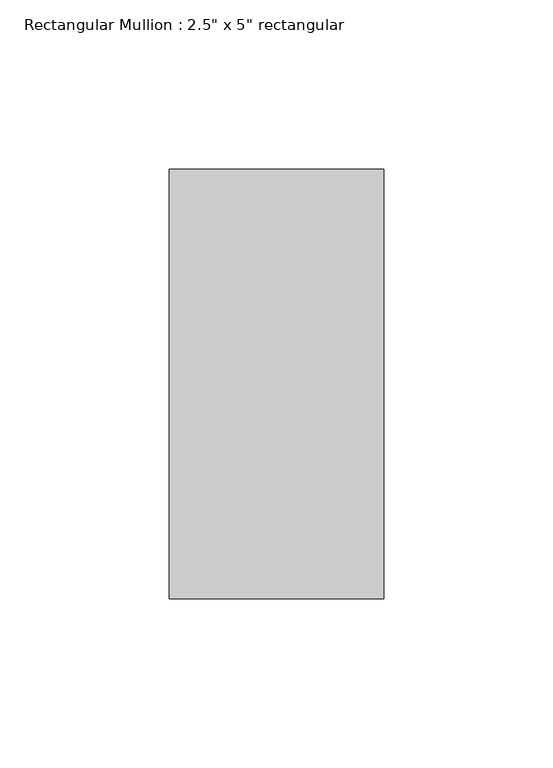
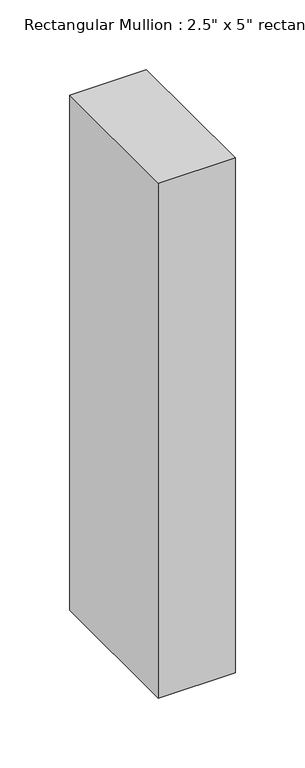
"""IFC4 building model written with IfcOpenShell, lengths in millimetres: member geometry."""

from ifc_helpers import new_model, si_unit, frame, origin, place, context, project, spatial, polyline, outline, extrude, source, transform, mapped, element, save


def member_24b1c93a(model_context):
    return source(origin(), model_context, "Body", "SweptSolid", [
        extrude(outline(polyline([(0.0, 63.5), (0.0, -63.5), (-63.5, -63.5), (-63.5, 63.5), (0.0, 63.5)])), frame((0.0, 0.0, -450.8169271), z_axis=(0.0, 0.0, 1.0), x_axis=(1.0, 0.0, 0.0)), (0.0, 0.0, 1.0), 450.8169271),
    ])


if __name__ == "__main__":
    model = new_model("IFC4")
    model_context = context("Model", 3, world=origin())
    ifc_project = project(units=[si_unit("LENGTHUNIT", "METRE", prefix="MILLI")], contexts=[model_context])
    site = spatial("IfcSite", under=ifc_project)
    building = spatial("IfcBuilding", under=site)
    placement = place(None, origin())
    member_shape = member_24b1c93a(model_context)
    element("IfcMember", 1, ObjectType="Rectangular Mullion : 2.5\" x 5\" rectangular", at=placement, inside=building, context=model_context, shape_type="MappedRepresentation", body=[
        mapped(member_shape, transform((0.0, 0.0, 0.0), x_axis=(1.0, 0.0, 0.0), y_axis=(0.0, 1.0, 0.0), z_axis=(0.0, 0.0, 1.0))),
    ])
    save(model, "model.ifc")

# Revit data of these elements
# Type "Rectangular Mullion : 2.5\" x 5\" rectangular"
#   built-in parameter 1007304 = 0.416667 (stored number, unit not read)
#   built-in parameter 1007301 = 0.104167 (stored number, unit not read)
#   built-in parameter 1007300 = 0.104167 (stored number, unit not read)
# Element 1 (IfcMember, "Rectangular Mullion : 2.5\" x 5\" rectangular")
#   Materials on its faces: "Aluminum"
# Materials
#   "Aluminum": class "Metal", colour RGB 247 247 247, transparency 0, Description = "Aluminum 6061", Cost = 0
